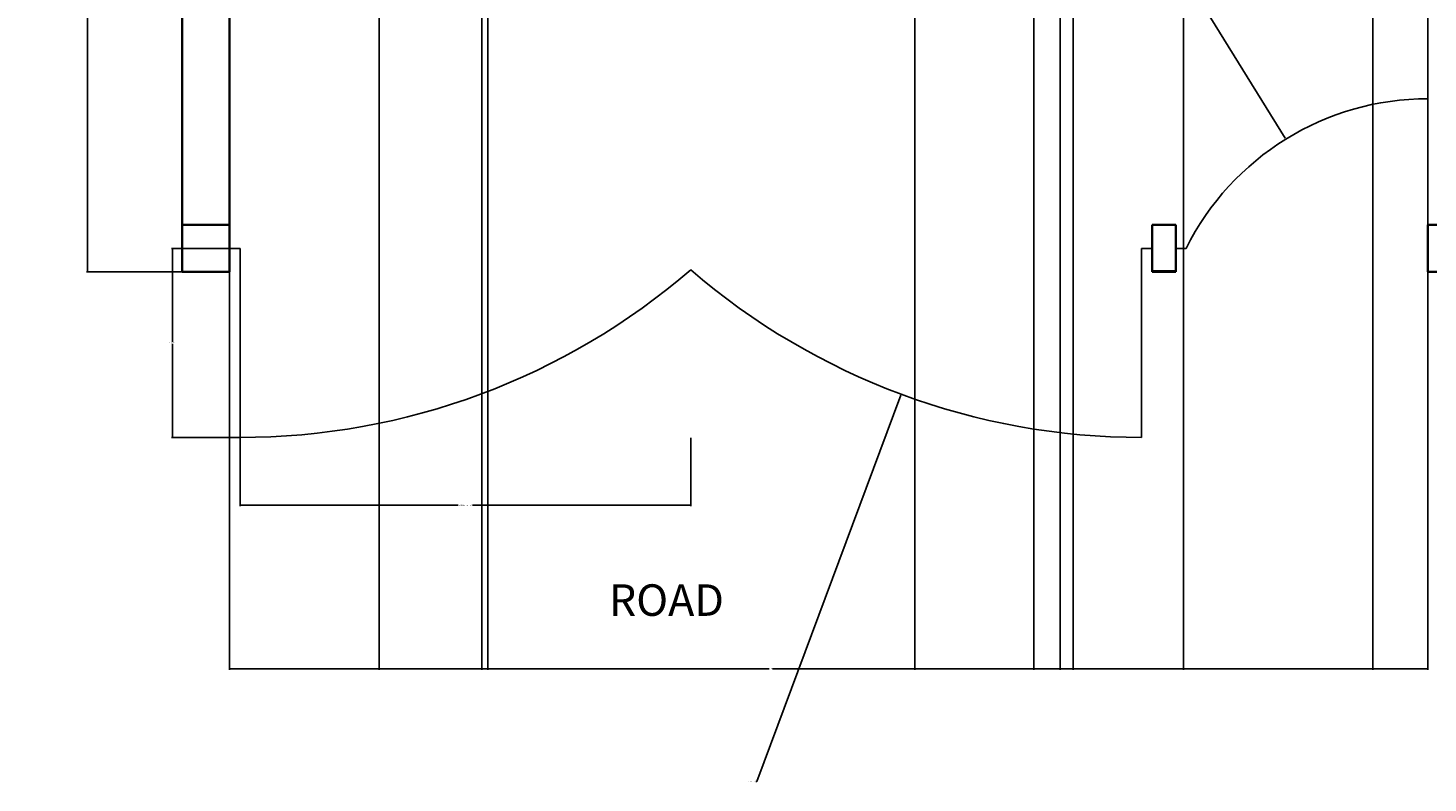
# Model space of a CAD drawing. Units: inches. Extents: x -10 to 502, y -868 to 56.
# Tile 1 of 14: x 6 to 272, y -868 to -724. Entities that reach past the tile are written whole.
import ezdxf

# ---------------------------------------------------------------- set-up
doc = ezdxf.new("R2010")
doc.units = ezdxf.units.IN
doc.header["$MEASUREMENT"] = 0
for name, color, linetype, lineweight in [('A-ANNO-DIMS', 2, 'Continuous', 18), ('A-ANNO-TEXT', 7, 'Continuous', 18), ('A-WALL', 7, 'Continuous', 35), ('L-GATE', 4, 'Continuous', 25), ('L-WALL', 7, 'Continuous', 35)]:
    doc.layers.add(name, color=color, linetype=linetype, lineweight=lineweight)
doc.styles.get("Standard").update_dxf_attribs({"font": 'arial.ttf'})
doc.dimstyles.get("Standard").update_dxf_attribs({"dimtxt": 0.18, "dimasz": 0.18, "dimexe": 0.18, "dimexo": 0.0625, "dimgap": 0.09, "dimtad": 0, "dimtih": 1, "dimtoh": 1, "dimdec": 0, "dimzin": 0, "dimdsep": 46, "dimlunit": 3, "dimtxsty": 'Standard', "dimcen": 0.09, "dimadec": 0, "dimazin": 0, "dimtfac": 1, "dimtdec": 0, "dimtofl": 0, "dimtmove": 0, "dimatfit": 3, "dimfxl": 1, "dimtolj": 1, "dimtzin": 0, "dimarcsym": 0})

# ---------------------------------------------------------------- blocks, each defined once
blk = doc.blocks.new('*D2')
at = {"layer": 'A-ANNO-DIMS', "color": 0, "lineweight": -2, "transparency": 16777216}
for p, q in [((34.89, 12.15), (16.75, 12.15)), ((16.93, 11.97), (16.93, -376.2)), ((16.93, -770.67), (16.93, -382.51)), ((34.89, -770.85), (16.75, -770.85))]:
    blk.add_line(p, q, dxfattribs=at)
at = {"layer": 'A-ANNO-DIMS', "color": 0, "transparency": 16777216}
for points in [[(16.9, 11.97), (16.96, 11.97), (16.93, 12.15)], [(16.9, -770.67), (16.96, -770.67), (16.93, -770.85)]]:
    blk.add_solid(points, dxfattribs=at)
at = {"layer": 'Defpoints', "color": 0, "transparency": 16777216}
for p in [(34.95, 12.15), (16.93, -770.85), (34.95, -770.85)]:
    blk.add_point(p, dxfattribs=at)
at = {"layer": 'A-ANNO-DIMS', "color": 0, "transparency": 16777216, "insert": (16.93, -379.35), "char_height": 6, "attachment_point": 5}
blk.add_mtext('\\A1;65\'-3"', dxfattribs=at)
blk = doc.blocks.new('GATE-DRIVE-LEAF')
blk.add_line((85.75, 36), (85.75, 0))
blk.add_arc((85.75, 131.15), 131.15, 229.1677, 270)
blk = doc.blocks.new('*D27')
at = {"layer": 'A-ANNO-DIMS', "color": 0, "lineweight": -2, "transparency": 16777216}
for p, q in [((45.95, -802.42), (45.95, -815.4)), ((131.7, -802.42), (131.7, -815.4)), ((46.13, -815.22), (87.46, -815.22)), ((131.52, -815.22), (90.19, -815.22))]:
    blk.add_line(p, q, dxfattribs=at)
at = {"layer": 'A-ANNO-DIMS', "color": 0, "transparency": 16777216}
for points in [[(46.13, -815.19), (46.13, -815.25), (45.95, -815.22)], [(131.52, -815.19), (131.52, -815.25), (131.7, -815.22)]]:
    blk.add_solid(points, dxfattribs=at)
at = {"layer": 'Defpoints', "color": 0, "transparency": 16777216}
for p in [(45.95, -802.35), (131.7, -802.35), (45.95, -815.22)]:
    blk.add_point(p, dxfattribs=at)
at = {"layer": 'A-ANNO-DIMS', "color": 0, "transparency": 16777216, "insert": (88.83, -815.22), "char_height": 0.18, "attachment_point": 5}
blk.add_mtext('\\A1;GATE LEAF 7\'-2" TYP.', dxfattribs=at)
blk = doc.blocks.new('*D28')
at = {"layer": 'A-ANNO-DIMS', "color": 0, "lineweight": -2, "transparency": 16777216}
for p, q in [((45.89, -766.35), (32.91, -766.35)), ((33.09, -766.53), (33.09, -784.17)), ((33.09, -802.17), (33.09, -784.53)), ((45.89, -802.35), (32.91, -802.35))]:
    blk.add_line(p, q, dxfattribs=at)
at = {"layer": 'A-ANNO-DIMS', "color": 0, "transparency": 16777216}
for points in [[(33.06, -766.53), (33.12, -766.53), (33.09, -766.35)], [(33.06, -802.17), (33.12, -802.17), (33.09, -802.35)]]:
    blk.add_solid(points, dxfattribs=at)
at = {"layer": 'Defpoints', "color": 0, "transparency": 16777216}
for p in [(33.09, -766.35), (45.95, -766.35), (45.95, -802.35)]:
    blk.add_point(p, dxfattribs=at)
at = {"layer": 'A-ANNO-DIMS', "color": 0, "transparency": 16777216, "insert": (33.09, -784.35), "char_height": 0.18, "attachment_point": 5}
blk.add_mtext('\\A1;3\'-0" TYP.', dxfattribs=at)
blk = doc.blocks.new('*D45')
at = {"layer": 'A-ANNO-DIMS', "color": 0, "lineweight": -2, "transparency": 16777216}
for p, q in [((196.98, -587.92), (196.98, -846.58)), ((271.95, -587.92), (271.95, -846.58)), ((197.16, -846.4), (234.14, -846.4)), ((271.77, -846.4), (234.8, -846.4))]:
    blk.add_line(p, q, dxfattribs=at)
at = {"layer": 'A-ANNO-DIMS', "color": 0, "transparency": 16777216}
for points in [[(197.16, -846.37), (197.16, -846.43), (196.98, -846.4)], [(271.77, -846.37), (271.77, -846.43), (271.95, -846.4)]]:
    blk.add_solid(points, dxfattribs=at)
at = {"layer": 'Defpoints', "color": 0, "transparency": 16777216}
for p in [(196.98, -587.85), (271.95, -587.85), (271.95, -846.4)]:
    blk.add_point(p, dxfattribs=at)
at = {"layer": 'A-ANNO-DIMS', "color": 0, "transparency": 16777216, "insert": (234.47, -846.4), "char_height": 0.18, "attachment_point": 5}
blk.add_mtext('\\A1;6\'-3"', dxfattribs=at)
blk = doc.blocks.new('*D47')
at = {"layer": 'A-ANNO-DIMS', "color": 0, "lineweight": -2, "transparency": 16777216}
for p, q in [((91.95, -494.92), (91.95, -846.58)), ((201.95, -494.92), (201.95, -846.58)), ((92.13, -846.4), (146.62, -846.4)), ((201.77, -846.4), (147.28, -846.4))]:
    blk.add_line(p, q, dxfattribs=at)
at = {"layer": 'A-ANNO-DIMS', "color": 0, "transparency": 16777216}
for points in [[(92.13, -846.37), (92.13, -846.43), (91.95, -846.4)], [(201.77, -846.37), (201.77, -846.43), (201.95, -846.4)]]:
    blk.add_solid(points, dxfattribs=at)
at = {"layer": 'Defpoints', "color": 0, "transparency": 16777216}
for p in [(91.95, -494.85), (201.95, -494.85), (201.95, -846.4)]:
    blk.add_point(p, dxfattribs=at)
at = {"layer": 'A-ANNO-DIMS', "color": 0, "transparency": 16777216, "insert": (146.95, -846.4), "char_height": 0.18, "attachment_point": 5}
blk.add_mtext('\\A1;9\'-2"', dxfattribs=at)
blk = doc.blocks.new('*D48')
at = {"layer": 'A-ANNO-DIMS', "color": 0, "lineweight": -2, "transparency": 16777216}
for p, q in [((43.95, -332.92), (43.95, -846.58)), ((72.45, -332.92), (72.45, -846.58)), ((44.13, -846.4), (57.66, -846.4)), ((72.27, -846.4), (58.74, -846.4))]:
    blk.add_line(p, q, dxfattribs=at)
at = {"layer": 'A-ANNO-DIMS', "color": 0, "transparency": 16777216}
for points in [[(44.13, -846.37), (44.13, -846.43), (43.95, -846.4)], [(72.27, -846.37), (72.27, -846.43), (72.45, -846.4)]]:
    blk.add_solid(points, dxfattribs=at)
at = {"layer": 'Defpoints', "color": 0, "transparency": 16777216}
for p in [(43.95, -332.85), (72.45, -332.85), (72.45, -846.4)]:
    blk.add_point(p, dxfattribs=at)
at = {"layer": 'A-ANNO-DIMS', "color": 0, "transparency": 16777216, "insert": (58.2, -846.4), "char_height": 0.18, "attachment_point": 5}
blk.add_mtext('\\A1;2\'-4 1/2"', dxfattribs=at)
blk = doc.blocks.new('*D53')
at = {"layer": 'A-ANNO-DIMS', "color": 0, "lineweight": -2, "transparency": 16777216}
for p, q in [((174.32, -443.06), (174.32, -846.58)), ((204.45, -443.92), (204.45, -846.58)), ((174.5, -846.4), (189.05, -846.4)), ((204.27, -846.4), (189.72, -846.4))]:
    blk.add_line(p, q, dxfattribs=at)
at = {"layer": 'A-ANNO-DIMS', "color": 0, "transparency": 16777216}
for points in [[(174.5, -846.37), (174.5, -846.43), (174.32, -846.4)], [(204.27, -846.37), (204.27, -846.43), (204.45, -846.4)]]:
    blk.add_solid(points, dxfattribs=at)
at = {"layer": 'Defpoints', "color": 0, "transparency": 16777216}
for p in [(174.32, -443), (204.45, -443.85), (204.45, -846.4)]:
    blk.add_point(p, dxfattribs=at)
at = {"layer": 'A-ANNO-DIMS', "color": 0, "transparency": 16777216, "insert": (189.39, -846.4), "char_height": 0.18, "attachment_point": 5}
blk.add_mtext('\\A1;2\'-6"', dxfattribs=at)
blk = doc.blocks.new('*D56')
at = {"layer": 'A-ANNO-DIMS', "color": 0, "lineweight": -2, "transparency": 16777216}
for p, q in [((43.95, -549.92), (43.95, -846.58)), ((93.07, -549.92), (93.07, -846.58)), ((44.13, -846.4), (68.18, -846.4)), ((92.89, -846.4), (68.84, -846.4))]:
    blk.add_line(p, q, dxfattribs=at)
at = {"layer": 'A-ANNO-DIMS', "color": 0, "transparency": 16777216}
for points in [[(44.13, -846.37), (44.13, -846.43), (43.95, -846.4)], [(92.89, -846.37), (92.89, -846.43), (93.07, -846.4)]]:
    blk.add_solid(points, dxfattribs=at)
at = {"layer": 'Defpoints', "color": 0, "transparency": 16777216}
for p in [(43.95, -549.85), (93.07, -549.85), (43.95, -846.4)]:
    blk.add_point(p, dxfattribs=at)
at = {"layer": 'A-ANNO-DIMS', "color": 0, "transparency": 16777216, "insert": (68.51, -846.4), "char_height": 0.18, "attachment_point": 5}
blk.add_mtext('\\A1;4\'-1"', dxfattribs=at)
blk = doc.blocks.new('*D65')
at = {"layer": 'A-ANNO-DIMS', "color": 0, "lineweight": -2, "transparency": 16777216}
for p, q in [((225.45, -263.92), (225.45, -846.58)), ((261.45, -263.92), (261.45, -846.58)), ((225.63, -846.4), (243.12, -846.4)), ((261.27, -846.4), (243.78, -846.4))]:
    blk.add_line(p, q, dxfattribs=at)
at = {"layer": 'A-ANNO-DIMS', "color": 0, "transparency": 16777216}
for points in [[(225.63, -846.37), (225.63, -846.43), (225.45, -846.4)], [(261.27, -846.37), (261.27, -846.43), (261.45, -846.4)]]:
    blk.add_solid(points, dxfattribs=at)
at = {"layer": 'Defpoints', "color": 0, "transparency": 16777216}
for p in [(225.45, -263.85), (261.45, -263.85), (261.45, -846.4)]:
    blk.add_point(p, dxfattribs=at)
at = {"layer": 'A-ANNO-DIMS', "color": 0, "transparency": 16777216, "insert": (243.45, -846.4), "char_height": 0.18, "attachment_point": 5}
blk.add_mtext('\\A1;3\'-0"', dxfattribs=at)
blk = doc.blocks.new('*D66')
at = {"layer": 'A-ANNO-DIMS', "color": 0, "lineweight": -2, "transparency": 16777216}
for p, q in [((217.45, -671.3), (217.45, -671.12)), ((217.36, -671.21), (217.54, -671.21)), ((144.25, -867.86), (171.64, -794.28)), ((144.07, -867.86), (144.25, -867.86))]:
    blk.add_line(p, q, dxfattribs=at)
at = {"layer": 'A-ANNO-DIMS', "color": 0, "transparency": 16777216}
blk.add_solid([(171.61, -794.27), (171.67, -794.29), (171.7, -794.11)], dxfattribs=at)
at = {"layer": 'Defpoints', "color": 0, "transparency": 16777216}
for p in [(217.45, -671.21), (171.7, -794.11)]:
    blk.add_point(p, dxfattribs=at)
at = {"layer": 'A-ANNO-DIMS', "color": 0, "transparency": 16777216, "insert": (143.32, -867.86), "char_height": 0.18, "attachment_point": 5}
blk.add_mtext('\\A1;2X R10\'-11"', dxfattribs=at)
blk = doc.blocks.new('*D67')
at = {"layer": 'A-ANNO-DIMS', "color": 0, "lineweight": -2, "transparency": 16777216}
for p, q in [((228.48, -719.35), (228.66, -719.35)), ((228.66, -719.35), (244.8, -745.4)), ((271.86, -789.23), (272.04, -789.23)), ((271.95, -789.32), (271.95, -789.14))]:
    blk.add_line(p, q, dxfattribs=at)
at = {"layer": 'A-ANNO-DIMS', "color": 0, "transparency": 16777216}
blk.add_solid([(244.82, -745.39), (244.77, -745.42), (244.89, -745.56)], dxfattribs=at)
at = {"layer": 'Defpoints', "color": 0, "transparency": 16777216}
for p in [(244.89, -745.56), (271.95, -789.23)]:
    blk.add_point(p, dxfattribs=at)
at = {"layer": 'A-ANNO-DIMS', "color": 0, "transparency": 16777216, "insert": (227.85, -719.35), "char_height": 0.18, "attachment_point": 5}
blk.add_mtext('\\A1;R4\'-3 1/2"', dxfattribs=at)

msp = doc.modelspace()

# ---------------------------------------------------------------- linework, layer by layer
at = {"layer": 'A-WALL'}
msp.add_line((34.95, 12.15), (34.95, -770.85), dxfattribs=at)
at = {"layer": 'L-GATE'}
for p, q in [((271.95, -761.85), (271.95, -737.85)), ((43.95, -766.35), (45.95, -766.35)), ((219.45, -766.35), (217.45, -766.35)), ((223.95, -766.35), (225.95, -766.35))]:
    msp.add_line(p, q, dxfattribs=at)
msp.add_arc((271.95, -789.23), 51.37, 90, 153.5618, dxfattribs=at)
at = {"layer": 'L-WALL'}
for p, q in [((43.95, -549.85), (43.95, -770.85)), ((34.95, -761.85), (43.95, -761.85)), ((223.95, -761.85), (219.45, -761.85)), ((219.45, -770.85), (219.45, -761.85)), ((223.95, -761.85), (223.95, -766.35)), ((271.95, -761.85), (271.95, -770.85)), ((271.95, -761.85), (453.45, -761.85)), ((223.95, -766.35), (223.95, -770.85)), ((34.95, -770.85), (43.95, -770.85)), ((223.95, -770.71), (219.45, -770.7)), ((223.95, -770.85), (219.45, -770.85)), ((271.95, -770.85), (457.95, -770.85))]:
    msp.add_line(p, q, dxfattribs=at)

# ---------------------------------------------------------------- block references
at = {"layer": 'L-GATE', "extrusion": (0, 0, -1), "zscale": -1}
msp.add_blockref('GATE-DRIVE-LEAF', (-131.7, -802.35), dxfattribs=at)
at = {"layer": 'L-GATE'}
msp.add_blockref('GATE-DRIVE-LEAF', (131.7, -802.35), dxfattribs=at)

# ---------------------------------------------------------------- texts
at = {"layer": 'A-ANNO-TEXT', "insert": (116.13, -830.31), "char_height": 6, "attachment_point": 1}
msp.add_mtext('ROAD', dxfattribs=at)

# ---------------------------------------------------------------- dimensions: what is measured, and where the dimension line sits
at = {"layer": 'A-ANNO-DIMS'}
dim = msp.add_linear_dim(base=(16.93, -770.85), p1=(34.95, 12.15), p2=(34.95, -770.85), angle=90, dimstyle='Standard', override={"dimtxt": 6, "dimclrd": 0, "dimclre": 0, "dimclrt": 0}, dxfattribs=at)
dim.commit()
dim.dimension.update_dxf_attribs({"geometry": '*D2', "text_midpoint": (16.93, -379.35)})
for base, p1, p2, picture, middle in [((261.45, -846.4), (225.45, -263.85), (261.45, -263.85), '*D65', (243.45, -846.4)), ((72.45, -846.4), (43.95, -332.85), (72.45, -332.85), '*D48', (58.2, -846.4)), ((204.45, -846.4), (174.32, -443), (204.45, -443.85), '*D53', (189.39, -846.4)), ((201.95, -846.4), (91.95, -494.85), (201.95, -494.85), '*D47', (146.95, -846.4)), ((43.95, -846.4), (93.07, -549.85), (43.95, -549.85), '*D56', (68.51, -846.4)), ((271.95, -846.4), (196.98, -587.85), (271.95, -587.85), '*D45', (234.47, -846.4))]:
    dim = msp.add_linear_dim(base=base, p1=p1, p2=p2, dimstyle='Standard', override={"dimdec": 1, "dimlfac": 1, "dimrnd": 0, "dimzin": 1, "dimdsep": 46, "dimlunit": 4, "dimfrac": 2}, dxfattribs=at)
    dim.commit()
    dim.dimension.update_dxf_attribs({"geometry": picture, "text_midpoint": middle})
dim = msp.add_radius_dim(center=(217.45, -671.21), mpoint=(171.7, -794.11), text='2X <>', dimstyle='Standard', override={"dimdec": 1, "dimlfac": 1, "dimrnd": 0, "dimzin": 1, "dimdsep": 46, "dimlunit": 4, "dimfrac": 2}, dxfattribs=at)
dim.commit()
dim.dimension.update_dxf_attribs({"geometry": '*D66', "text_midpoint": (143.32, -867.86), "dimtype": 164})
dim = msp.add_radius_dim(center=(271.95, -789.23), mpoint=(244.89, -745.56), dimstyle='Standard', override={"dimdec": 1, "dimlfac": 1, "dimrnd": 0, "dimzin": 1, "dimdsep": 46, "dimlunit": 4, "dimfrac": 2}, dxfattribs=at)
dim.commit()
dim.dimension.update_dxf_attribs({"geometry": '*D67', "text_midpoint": (227.85, -719.35), "dimtype": 164})
for base, p1, p2, angle, text, picture, middle in [((33.09, -766.35), (45.95, -802.35), (45.95, -766.35), 90, '<> TYP.', '*D28', (33.09, -784.35)), ((45.95091602, -815.21523663), (131.70091602, -802.35273663), (45.95091602, -802.35273663), 180, 'GATE LEAF <> TYP.', '*D27', (88.82591602, -815.21523663))]:
    dim = msp.add_linear_dim(base=base, p1=p1, p2=p2, angle=angle, text=text, dimstyle='Standard', override={"dimdec": 1, "dimlfac": 1, "dimrnd": 0, "dimzin": 1, "dimdsep": 46, "dimlunit": 4, "dimfrac": 2}, dxfattribs=at)
    dim.commit()
    dim.dimension.update_dxf_attribs({"geometry": picture, "text_midpoint": middle})

doc.saveas('drawing.dxf')
